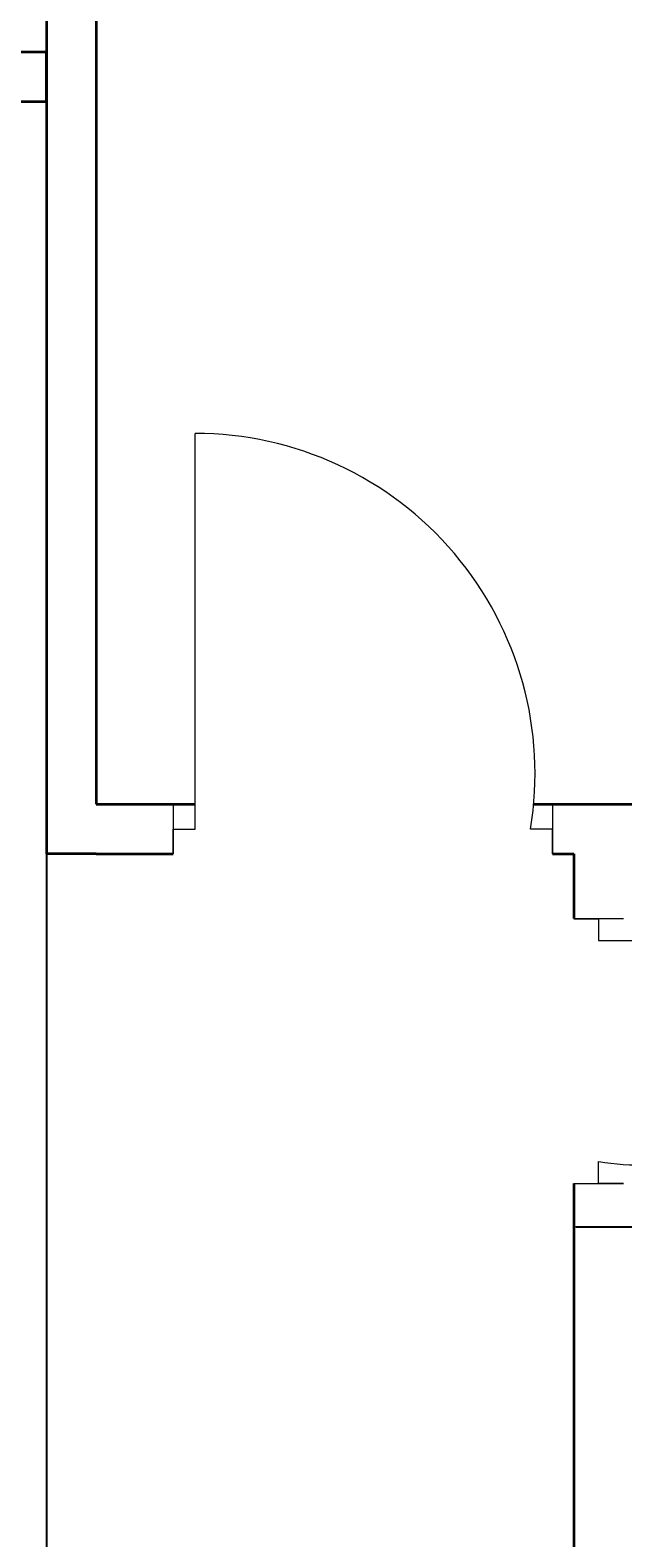
# Model space of a CAD drawing. Units: inches. Extents: x 1088 to 1703, y 668 to 1875.
# Tile 33 of 45: x 1436 to 1490, y 1606 to 1743. Entities that reach past the tile are written whole.
import ezdxf

# ---------------------------------------------------------------- set-up
doc = ezdxf.new("R2010")
doc.units = ezdxf.units.IN
for name, color, linetype, lineweight in [('A-ANNO-DIMS', 2, 'Continuous', 18), ('A-DOOR', 4, 'Continuous', 18), ('A-WALL', 7, 'Continuous', 35)]:
    doc.layers.add(name, color=color, linetype=linetype, lineweight=lineweight)
doc.styles.get("Standard").update_dxf_attribs({"font": 'arial.ttf'})
doc.dimstyles.get("Standard").update_dxf_attribs({"dimtxt": 0.18, "dimasz": 0.18, "dimexe": 0.18, "dimexo": 0.0625, "dimgap": 0.09, "dimtad": 0, "dimtih": 1, "dimtoh": 1, "dimdec": 4, "dimzin": 0, "dimdsep": 46, "dimtxsty": 'Standard', "dimcen": 0.09, "dimadec": 0, "dimazin": 0, "dimtfac": 1, "dimtdec": 4, "dimtofl": 0, "dimtmove": 0, "dimatfit": 3, "dimfxl": 1, "dimtolj": 1, "dimtzin": 0, "dimarcsym": 0})

# ---------------------------------------------------------------- blocks, each defined once
blk = doc.blocks.new('DOOR-SWING-24')
for p, q in [((4.5, 24.09), (0, 24.09)), ((0, 24.09), (2.25, 24.09)), ((2.25, 24.09), (2.25, 22.09)), ((2.25, 22.09), (26.25, 22.09)), ((2.25, 0), (2.25, 2)), ((0, 0), (4.5, 0)), ((4.5, 0), (2.25, 0))]:
    blk.add_line(p, q)
blk.add_arc((5.84, 22.09), 20.41, 259.876, 0)
blk = doc.blocks.new('*D24')
at = {"layer": 'A-ANNO-DIMS', "color": 0, "lineweight": -2, "transparency": 16777216}
for p, q in [((1485.34, 1638.5), (1485.34, 1634.44)), ((1511.59, 1638.5), (1511.59, 1634.44)), ((1485.52, 1634.62), (1497.53, 1634.62)), ((1511.41, 1634.62), (1499.41, 1634.62))]:
    blk.add_line(p, q, dxfattribs=at)
at = {"layer": 'A-ANNO-DIMS', "color": 0, "transparency": 16777216}
for points in [[(1485.52, 1634.65), (1485.52, 1634.59), (1485.34, 1634.62)], [(1511.41, 1634.65), (1511.41, 1634.59), (1511.59, 1634.62)]]:
    blk.add_solid(points, dxfattribs=at)
at = {"layer": 'Defpoints', "color": 0, "transparency": 16777216}
for p in [(1485.34, 1638.56), (1511.59, 1638.56), (1511.59, 1634.62)]:
    blk.add_point(p, dxfattribs=at)
at = {"layer": 'A-ANNO-DIMS', "color": 0, "transparency": 16777216, "insert": (1498.47, 1634.62), "char_height": 0.18, "attachment_point": 5}
blk.add_mtext('\\A1;DOOR 26 TYP.', dxfattribs=at)
blk = doc.blocks.new('*D38')
at = {"layer": 'A-ANNO-DIMS', "color": 0, "lineweight": -2, "transparency": 16777216}
for p, q in [((1317.34, 1736.94), (1317.34, 725.55)), ((1437.34, 1736.94), (1437.34, 725.55)), ((1317.52, 725.73), (1377.06, 725.73)), ((1437.16, 725.73), (1377.62, 725.73))]:
    blk.add_line(p, q, dxfattribs=at)
at = {"layer": 'A-ANNO-DIMS', "color": 0, "transparency": 16777216}
for points in [[(1317.52, 725.76), (1317.52, 725.7), (1317.34, 725.73)], [(1437.16, 725.76), (1437.16, 725.7), (1437.34, 725.73)]]:
    blk.add_solid(points, dxfattribs=at)
at = {"layer": 'Defpoints', "color": 0, "transparency": 16777216}
for p in [(1317.34, 1737.01), (1437.34, 1737.01), (1437.34, 725.73)]:
    blk.add_point(p, dxfattribs=at)
at = {"layer": 'A-ANNO-DIMS', "color": 0, "transparency": 16777216, "insert": (1377.34, 725.73), "char_height": 0.18, "attachment_point": 5}
blk.add_mtext('\\A1;120', dxfattribs=at)

msp = doc.modelspace()

# ---------------------------------------------------------------- linework, layer by layer
at = {"layer": 'A-DOOR'}
for p, q in [((1450.857, 1670.808), (1450.857, 1706.808)), ((1448.857, 1673.058), (1448.857, 1668.558)), ((1483.393, 1673.058), (1483.393, 1668.558)), ((1448.857, 1668.558), (1448.857, 1670.808)), ((1448.857, 1670.808), (1450.857, 1670.808)), ((1483.393, 1670.808), (1481.393, 1670.808)), ((1483.393, 1668.558), (1483.393, 1670.808))]:
    msp.add_line(p, q, dxfattribs=at)
msp.add_arc((1450.857, 1675.857), 30.951, 350.61111, 90, dxfattribs=at)
at = {"layer": 'A-WALL'}
for p, q in [((1437.345, 1803.558), (1437.345, 1668.558)), ((1441.845, 1799.058), (1441.845, 1673.058)), ((1437.345, 1741.507), (1403.489, 1741.507)), ((1437.345, 1737.007), (1437.345, 1741.507)), ((1403.489, 1737.007), (1437.345, 1737.007)), ((1441.845, 1673.058), (1450.857, 1673.058)), ((1481.681, 1673.058), (1585.845, 1673.058)), ((1441.845, 1668.558), (1437.345, 1668.558)), ((1441.845, 1668.558), (1448.857, 1668.558)), ((1483.393, 1668.558), (1485.345, 1668.558)), ((1485.345, 1668.558), (1485.345, 1662.653)), ((1485.345, 1638.558), (1485.345, 1608.558)), ((1485.345, 1608.558), (1485.345, 1604.058))]:
    msp.add_line(p, q, dxfattribs=at)

# ---------------------------------------------------------------- block references
at = {"layer": 'A-DOOR'}
msp.add_blockref('DOOR-SWING-24', (1485.345, 1638.558), dxfattribs=at)

# ---------------------------------------------------------------- dimensions: what is measured, and where the dimension line sits
at = {"layer": 'A-ANNO-DIMS'}
dim = msp.add_linear_dim(base=(1437.345, 725.729), p1=(1317.345, 1737.007), p2=(1437.345, 1737.007), dimstyle='Standard', override={"dimdec": 0, "dimlfac": 1, "dimrnd": 0, "dimzin": 0, "dimdsep": 46, "dimlunit": 2}, dxfattribs=at)
dim.commit()
dim.dimension.update_dxf_attribs({"geometry": '*D38', "text_midpoint": (1377.345, 725.729)})
dim = msp.add_linear_dim(base=(1511.595, 1634.621), p1=(1485.345, 1638.558), p2=(1511.595, 1638.558), text='DOOR <> TYP.', dimstyle='Standard', override={"dimdec": 0, "dimlfac": 1, "dimrnd": 0, "dimzin": 0, "dimdsep": 46, "dimlunit": 2}, dxfattribs=at)
dim.commit()
dim.dimension.update_dxf_attribs({"geometry": '*D24', "text_midpoint": (1498.47, 1634.621)})

doc.saveas('drawing.dxf')
